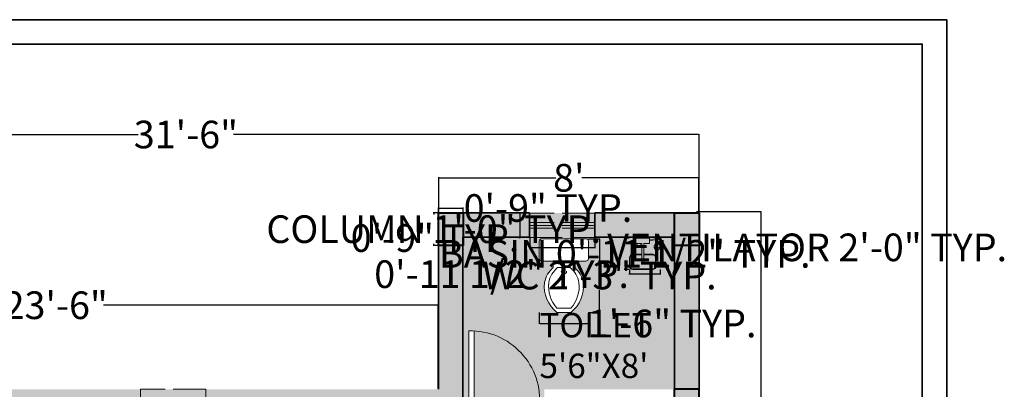
# Model space of a CAD drawing. Units: inches. Extents: x 1077 to 2505, y 1892 to 2728.
# Tile 18 of 26: x 1306 to 1669, y 2586 to 2722. Entities that reach past the tile are written whole.
import ezdxf

# ---------------------------------------------------------------- set-up
doc = ezdxf.new("R2010")
doc.units = ezdxf.units.IN
doc.linetypes.add('ACAD_ISO02W100', pattern=[15, 12, -3])
doc.layers.get('Defpoints').update_dxf_attribs({"color": 220, "linetype": 'ACAD_ISO02W100'})
for name, color, linetype, lineweight in [('A-ANNO-DIMS', 2, 'Continuous', 18), ('A-ANNO-TTLB', 7, 'Continuous', 35), ('A-AREA-IDEN', 7, 'Continuous', 18), ('A-COLS', 7, 'Continuous', 40), ('A-DOOR', 4, 'Continuous', 18), ('A-FLOR-FIXT', 8, 'Continuous', 13), ('A-GLAZ-VENT', 6, 'ACAD_ISO02W100', 13), ('A-WALL-PATT', 7, 'Continuous', 9), ('A_FUR 1', 5, 'Continuous', 5), ('WALL', 7, 'Continuous', 35)]:
    doc.layers.add(name, color=color, linetype=linetype, lineweight=lineweight)
doc.layers.add('A-FLOR-PATT', color=254, linetype='Continuous', lineweight=9, true_color=0xd7ebd2)
doc.styles.get("Standard").update_dxf_attribs({"font": 'arial.ttf'})
doc.dimstyles.get("Standard").update_dxf_attribs({"dimtxt": 10.18, "dimasz": 0.18, "dimexe": 0.18, "dimexo": 0.0625, "dimgap": 0.09, "dimtad": 0, "dimtih": 1, "dimtoh": 1, "dimdec": 0, "dimzin": 0, "dimdsep": 46, "dimlunit": 3, "dimtxsty": 'Standard', "dimcen": 0.09, "dimadec": 0, "dimazin": 0, "dimtfac": 1, "dimtdec": 0, "dimtofl": 0, "dimtmove": 0, "dimatfit": 3, "dimfxl": 1, "dimtolj": 1, "dimtzin": 0, "dimarcsym": 0})

# ---------------------------------------------------------------- blocks, each defined once
blk = doc.blocks.new('*D1')
at = {"layer": 'A-ANNO-DIMS', "color": 0, "lineweight": -2, "transparency": 16777216}
for p, q in [((1460.66, 2651.34), (1460.66, 2664.26)), ((1460.84, 2664.08), (1503.8, 2664.08)), ((1556.32, 2664.08), (1513.36, 2664.08)), ((1556.5, 2651.34), (1556.5, 2664.26))]:
    blk.add_line(p, q, dxfattribs=at)
at = {"layer": 'A-ANNO-DIMS', "color": 0, "transparency": 16777216}
for points in [[(1460.84, 2664.11), (1460.84, 2664.05), (1460.66, 2664.08)], [(1556.32, 2664.11), (1556.32, 2664.05), (1556.5, 2664.08)]]:
    blk.add_solid(points, dxfattribs=at)
at = {"layer": 'Defpoints', "color": 0, "transparency": 16777216}
for p in [(1556.5, 2664.08), (1460.66, 2651.28), (1556.5, 2651.28)]:
    blk.add_point(p, dxfattribs=at)
at = {"layer": 'A-ANNO-DIMS', "color": 0, "transparency": 16777216, "insert": (1508.58, 2664.08), "char_height": 10.18, "attachment_point": 5}
blk.add_mtext("\\A1;8'", dxfattribs=at)
blk = doc.blocks.new('ESTSET')
at = {"layer": 'A_FUR 1'}
for p, q in [((-10.44, 4.1), (-10.44, 32.1)), ((-8.44, 4.1), (-8.44, 32.1)), ((-36.44, 6.1), (-36.44, 3.1)), ((-34.44, 6.1), (-36.44, 6.1)), ((-34.44, 4.1), (-34.44, 6.1)), ((-34.44, 4.1), (-34.44, 6.1)), ((-32.44, 4.1), (-34.44, 4.1)), ((-32.44, 4.1), (-34.44, 4.1)), ((-32.44, 3.1), (-32.44, 4.1)), ((-10.44, 3.1), (-10.44, 4.1)), ((-10.44, 4.1), (-8.44, 4.1)), ((-10.44, 4.1), (-8.44, 4.1)), ((-8.44, 4.1), (-8.44, 6.1)), ((-8.44, 6.1), (-6.44, 6.1)), ((-8.44, 4.1), (-8.44, 6.1)), ((-6.44, 6.1), (-6.44, 3.1)), ((-6.44, 2.1), (-36.44, 2.1)), ((-35.44, 2.1), (-33.44, 2.1)), ((-7.44, 2.1), (-9.44, 2.1))]:
    blk.add_line(p, q, dxfattribs=at)
for points in [[(-21.44, 2.1), (-18.67, 2.1), (-18.67, 5.1), (-20.06, 5.1)], [(-20.06, 5.1), (-20.06, -0.91)], [(-21.44, 2.1), (-21.44, -0.91), (-20.06, -0.91)]]:
    blk.add_lwpolyline(points, dxfattribs=at)
for centre, radius, start, end in [((-8.91, 6.46), 25.64, 88.9606, 185.2816), ((-35.44, 3.1), 1, 180, 270), ((-33.44, 3.1), 1, 270, 0), ((-9.44, 3.1), 1, 180, 270), ((-7.44, 3.1), 1, 270, 0)]:
    blk.add_arc(centre, radius, start, end, dxfattribs=at)
blk = doc.blocks.new('A$C2AC94788')
for p, q in [((0, 0.505), (0, 0.665)), ((0.025, 0.69), (0.435, 0.69)), ((0.46, 0.665), (0.46, 0.505)), ((0.435, 0.48), (0.025, 0.48)), ((0.13, 0.48), (0.13, 0.42)), ((0.33, 0.42), (0.33, 0.48)), ((0.17, 0.42), (0.29, 0.42)), ((0.1641, 0.0392), (0.2959, 0.0392)), ((0.2291, 0.0392), (0.23, 0.0392)), ((0.2309, 0.0392), (0.23, 0.0392)), ((0.165, 0), (0.295, 0))]:
    blk.add_line(p, q)
for centre, radius, start, end in [((0.025, 0.665), 0.025, 90, 180), ((0.435, 0.665), 0.025, 0, 90), ((0.025, 0.505), 0.025, 180, 270), ((0.435, 0.505), 0.025, 270, 0), ((0.2874, 0.2356), 0.2425, 130.48854, 169.44501), ((0.3274, 0.2356), 0.2425, 130.48854, 169.44501), ((0.23, 0.385), 0.025, 180, 0), ((0.1326, 0.2356), 0.2425, 10.55499, 49.51146), ((0.1726, 0.2356), 0.2425, 10.55499, 49.51146), ((0.3601, 0.2448), 0.313, 173.53688, 231.44828), ((0.4001, 0.2448), 0.313, 173.53688, 221.06038), ((0.0999, 0.2448), 0.313, 308.55172, 6.46312), ((0.0599, 0.2448), 0.313, 318.93962, 6.46312)]:
    blk.add_arc(centre, radius, start, end)
blk = doc.blocks.new('A$C7A0926BE')
for p, q in [((-6.55, 0), (-5.57, 0)), ((-6.55, -0.65), (-6.55, 0)), ((-5.57, 0), (-5.57, -0.65)), ((-2.89, 0), (-2.89, -2.29)), ((2.89, 0), (-2.89, 0)), ((2.89, -2.29), (2.89, 0)), ((-7.32, -3.29), (-7.32, -3.94)), ((-5.57, -0.65), (-6.55, -0.65)), ((-6.34, -0.65), (-5.74, -0.65)), ((-6.34, -2.33), (-6.34, -0.65)), ((-5.74, -2.33), (-6.34, -2.33)), ((-5.74, -0.65), (-5.74, -2.33)), ((-5.57, -0.28), (-2.89, -0.56)), ((-5.57, -0.65), (-2.89, -0.94)), ((-4.84, -3.94), (-4.85, -3.29)), ((-2.89, -2.29), (-0.45, -2.29)), ((0.39, -2.29), (2.89, -2.29)), ((1.04, -2.29), (1.04, -3.12)), ((2.37, -2.29), (1.04, -2.29)), ((1.04, -3.12), (2.37, -3.12)), ((1.13, -3.12), (1.13, -3.23)), ((2.3, -3.12), (1.13, -3.12)), ((1.13, -3.23), (2.3, -3.23)), ((2.3, -3.23), (2.3, -3.12)), ((2.37, -3.12), (2.37, -2.29))]:
    blk.add_line(p, q)
at = {"ltscale": 100}
for p, q in [((-0.45, -10.48), (-0.45, -2.29)), ((0.39, -10.48), (0.39, -2.29)), ((0.18, -10.69), (-0.24, -10.69))]:
    blk.add_line(p, q, dxfattribs=at)
for points in [[(-0.45, -6.79), (-4.23, -6.79, 0.414214), (-5.63, -8.19), (-5.63, -11.8, 0.414214), (-4.23, -13.2), (4.17, -13.2, 0.414214), (5.57, -11.8), (5.57, -8.19, 0.414214), (4.17, -6.79), (0.39, -6.79)], [(-0.45, -7), (-4.23, -7, 0.414214), (-5.42, -8.19), (-5.42, -11.8, 0.414214), (-4.23, -12.99), (4.17, -12.99, 0.414214), (5.36, -11.8), (5.36, -8.19, 0.414214), (4.17, -7), (0.39, -7)]]:
    blk.add_lwpolyline(points, format="xyb", dxfattribs=at)
for centre, start, end in [((-0.24, -10.48), 180, 270), ((0.18, -10.48), 270, 0)]:
    blk.add_arc(centre, 0.21, start, end, dxfattribs=at)
at = {"extrusion": (0, 0, -1)}
blk.add_ellipse((-6.08, -3.29), major_axis=(-1.24, 0), ratio=0.790849, dxfattribs=at)
blk.add_ellipse((-6.08, -3.94), major_axis=(-1.24, 0), ratio=0.790849, start_param=3.141593, end_param=6.283185, dxfattribs=at)
blk = doc.blocks.new('C1')
h = blk.add_hatch(color=256)
h.dxf.hatch_style = 1
h.paths.add_polyline_path([(1668.56, 2445.41), (1677.56, 2445.41), (1677.56, 2457.41), (1668.56, 2457.41)])
for p, q in [((1668.56, 2457.41), (1677.56, 2457.41)), ((1668.56, 2445.41), (1668.56, 2457.41)), ((1677.56, 2457.41), (1677.56, 2445.41)), ((1677.56, 2445.41), (1668.56, 2445.41))]:
    blk.add_line(p, q)
blk = doc.blocks.new('*D13')
at = {"layer": 'A-ANNO-DIMS', "color": 0, "lineweight": -2, "transparency": 16777216}
for p, q in [((1178.64, 2586.44), (1178.64, 2617.31)), ((1178.82, 2617.13), (1301.91, 2617.13)), ((1460.32, 2617.13), (1337.23, 2617.13)), ((1460.5, 2586.44), (1460.5, 2617.31))]:
    blk.add_line(p, q, dxfattribs=at)
at = {"layer": 'A-ANNO-DIMS', "color": 0, "transparency": 16777216}
for points in [[(1178.82, 2617.16), (1178.82, 2617.1), (1178.64, 2617.13)], [(1460.32, 2617.16), (1460.32, 2617.1), (1460.5, 2617.13)]]:
    blk.add_solid(points, dxfattribs=at)
at = {"layer": 'Defpoints', "color": 0, "transparency": 16777216}
for p in [(1460.5, 2617.13), (1178.64, 2586.38), (1460.5, 2586.38)]:
    blk.add_point(p, dxfattribs=at)
at = {"layer": 'A-ANNO-DIMS', "color": 0, "transparency": 16777216, "insert": (1319.57, 2617.13), "char_height": 10.18, "attachment_point": 5}
blk.add_mtext('\\A1;23\'-6"', dxfattribs=at)
blk = doc.blocks.new('*D14')
at = {"layer": 'A-ANNO-DIMS', "color": 0, "lineweight": -2, "transparency": 16777216}
for p, q in [((1555.59, 2651.66), (1579.43, 2651.66)), ((1579.25, 2651.48), (1579.25, 2375.3)), ((1579.25, 2088.54), (1579.25, 2364.72)), ((1555.59, 2088.36), (1579.43, 2088.36))]:
    blk.add_line(p, q, dxfattribs=at)
at = {"layer": 'A-ANNO-DIMS', "color": 0, "transparency": 16777216}
for points in [[(1579.22, 2651.48), (1579.28, 2651.48), (1579.25, 2651.66)], [(1579.22, 2088.54), (1579.28, 2088.54), (1579.25, 2088.36)]]:
    blk.add_solid(points, dxfattribs=at)
at = {"layer": 'Defpoints', "color": 0, "transparency": 16777216}
for p in [(1555.53, 2651.66), (1555.53, 2088.36), (1579.25, 2088.36)]:
    blk.add_point(p, dxfattribs=at)
at = {"layer": 'A-ANNO-DIMS', "color": 0, "transparency": 16777216, "insert": (1579.25, 2370.01), "char_height": 10.18, "attachment_point": 5}
blk.add_mtext('\\A1;46\'-11"', dxfattribs=at)
blk = doc.blocks.new('VENT-24')
for p, q in [((3.5, 24), (3.5, 0)), ((4.5, 24), (4.5, 0)), ((5.5, 24), (5.5, 0))]:
    blk.add_line(p, q)
blk.add_lwpolyline([(0, 0), (9, 0), (9, 24), (0, 24)], close=True)
blk = doc.blocks.new('SHEET-FRAME-RESIDENTIAL')
for points in [[(0, 830.04), (543.52, 830.04), (543.52, 0), (0, 0)], [(9, 821.04), (534.52, 821.04), (534.52, 9), (9, 9)]]:
    blk.add_lwpolyline(points, close=True)
blk = doc.blocks.new('*D30')
at = {"layer": 'A-ANNO-DIMS', "color": 0, "lineweight": -2, "transparency": 16777216}
for p, q in [((1460.54, 2651.14), (1458.62, 2651.14)), ((1458.8, 2650.96), (1458.8, 2650.5)), ((1460.54, 2639.14), (1458.62, 2639.14)), ((1458.8, 2639.32), (1458.8, 2639.78))]:
    blk.add_line(p, q, dxfattribs=at)
at = {"layer": 'A-ANNO-DIMS', "color": 0, "transparency": 16777216}
for points in [[(1458.77, 2650.96), (1458.83, 2650.96), (1458.8, 2651.14)], [(1458.77, 2639.32), (1458.83, 2639.32), (1458.8, 2639.14)]]:
    blk.add_solid(points, dxfattribs=at)
at = {"layer": 'Defpoints', "color": 0, "transparency": 16777216}
for p in [(1458.8, 2651.14), (1460.6, 2651.14), (1460.6, 2639.14)]:
    blk.add_point(p, dxfattribs=at)
at = {"layer": 'A-ANNO-DIMS', "color": 0, "transparency": 16777216, "insert": (1458.8, 2645.14), "char_height": 10.18, "attachment_point": 5}
blk.add_mtext('\\A1;COLUMN 1\'-0" TYP.', dxfattribs=at)
blk = doc.blocks.new('*D31')
at = {"layer": 'A-ANNO-DIMS', "color": 0, "lineweight": -2, "transparency": 16777216}
for p, q in [((1460.6, 2651.2), (1460.6, 2653.12)), ((1460.78, 2652.94), (1469.42, 2652.94)), ((1469.6, 2651.2), (1469.6, 2653.12)), ((1469.6, 2652.94), (1469.78, 2652.94))]:
    blk.add_line(p, q, dxfattribs=at)
at = {"layer": 'A-ANNO-DIMS', "color": 0, "transparency": 16777216}
for points in [[(1460.78, 2652.97), (1460.78, 2652.91), (1460.6, 2652.94)], [(1469.42, 2652.97), (1469.42, 2652.91), (1469.6, 2652.94)]]:
    blk.add_solid(points, dxfattribs=at)
at = {"layer": 'Defpoints', "color": 0, "transparency": 16777216}
for p in [(1469.6, 2652.94), (1460.6, 2651.14), (1469.6, 2651.14)]:
    blk.add_point(p, dxfattribs=at)
at = {"layer": 'A-ANNO-DIMS', "color": 0, "transparency": 16777216, "insert": (1500.89, 2652.94), "char_height": 10.18, "attachment_point": 5}
blk.add_mtext('\\A1;0\'-9" TYP.', dxfattribs=at)
blk = doc.blocks.new('*D42')
at = {"layer": 'A-ANNO-DIMS', "color": 0, "lineweight": -2, "transparency": 16777216}
for p, q in [((1515.87, 2641.64), (1520.06, 2641.64)), ((1519.88, 2641.46), (1519.88, 2633.41)), ((1519.88, 2614.65), (1519.88, 2622.7)), ((1515.87, 2614.47), (1520.06, 2614.47))]:
    blk.add_line(p, q, dxfattribs=at)
at = {"layer": 'A-ANNO-DIMS', "color": 0, "transparency": 16777216}
for points in [[(1519.85, 2641.46), (1519.91, 2641.46), (1519.88, 2641.64)], [(1519.85, 2614.65), (1519.91, 2614.65), (1519.88, 2614.47)]]:
    blk.add_solid(points, dxfattribs=at)
at = {"layer": 'Defpoints', "color": 0, "transparency": 16777216}
for p in [(1515.81, 2641.64), (1519.88, 2641.64), (1515.81, 2614.47)]:
    blk.add_point(p, dxfattribs=at)
at = {"layer": 'A-ANNO-DIMS', "color": 0, "transparency": 16777216, "insert": (1519.88, 2628.06), "char_height": 10.18, "attachment_point": 5}
blk.add_mtext('\\A1;WC 2\'-3" TYP.', dxfattribs=at)
blk = doc.blocks.new('*D43')
at = {"layer": 'A-ANNO-DIMS', "color": 0, "lineweight": -2, "transparency": 16777216}
for p, q in [((1497.7, 2614.41), (1497.7, 2610.22)), ((1515.81, 2614.41), (1515.81, 2610.22)), ((1497.88, 2610.4), (1515.63, 2610.4)), ((1515.81, 2610.4), (1515.99, 2610.4))]:
    blk.add_line(p, q, dxfattribs=at)
at = {"layer": 'A-ANNO-DIMS', "color": 0, "transparency": 16777216}
for points in [[(1497.88, 2610.43), (1497.88, 2610.37), (1497.7, 2610.4)], [(1515.63, 2610.43), (1515.63, 2610.37), (1515.81, 2610.4)]]:
    blk.add_solid(points, dxfattribs=at)
at = {"layer": 'Defpoints', "color": 0, "transparency": 16777216}
for p in [(1497.7, 2614.47), (1515.81, 2614.47), (1515.81, 2610.4)]:
    blk.add_point(p, dxfattribs=at)
at = {"layer": 'A-ANNO-DIMS', "color": 0, "transparency": 16777216, "insert": (1546.63, 2610.4), "char_height": 10.18, "attachment_point": 5}
blk.add_mtext('\\A1;1\'-6" TYP.', dxfattribs=at)
blk = doc.blocks.new('*D52')
at = {"layer": 'A-ANNO-DIMS', "color": 0, "lineweight": -2, "transparency": 16777216}
for p, q in [((1530.85, 2641.82), (1529, 2641.82)), ((1529.18, 2641.64), (1529.18, 2641.42)), ((1530.85, 2630.3), (1529, 2630.3)), ((1529.18, 2630.48), (1529.18, 2630.71))]:
    blk.add_line(p, q, dxfattribs=at)
at = {"layer": 'A-ANNO-DIMS', "color": 0, "transparency": 16777216}
for points in [[(1529.15, 2641.64), (1529.21, 2641.64), (1529.18, 2641.82)], [(1529.15, 2630.48), (1529.21, 2630.48), (1529.18, 2630.3)]]:
    blk.add_solid(points, dxfattribs=at)
at = {"layer": 'Defpoints', "color": 0, "transparency": 16777216}
for p in [(1529.18, 2641.82), (1530.91, 2641.82), (1530.91, 2630.3)]:
    blk.add_point(p, dxfattribs=at)
at = {"layer": 'A-ANNO-DIMS', "color": 0, "transparency": 16777216, "insert": (1529.18, 2636.06), "char_height": 10.18, "attachment_point": 5}
blk.add_mtext('\\A1;BASIN 0\'-11 1/2" TYP.', dxfattribs=at)
blk = doc.blocks.new('*D53')
at = {"layer": 'A-ANNO-DIMS', "color": 0, "lineweight": -2, "transparency": 16777216}
for p, q in [((1530.91, 2630.24), (1530.91, 2628.39)), ((1542.17, 2630.24), (1542.17, 2628.39)), ((1530.91, 2628.57), (1530.73, 2628.57)), ((1541.99, 2628.57), (1531.09, 2628.57))]:
    blk.add_line(p, q, dxfattribs=at)
at = {"layer": 'A-ANNO-DIMS', "color": 0, "transparency": 16777216}
for points in [[(1531.09, 2628.6), (1531.09, 2628.54), (1530.91, 2628.57)], [(1541.99, 2628.6), (1541.99, 2628.54), (1542.17, 2628.57)]]:
    blk.add_solid(points, dxfattribs=at)
at = {"layer": 'Defpoints', "color": 0, "transparency": 16777216}
for p in [(1530.91, 2630.3), (1542.17, 2630.3), (1530.91, 2628.57)]:
    blk.add_point(p, dxfattribs=at)
at = {"layer": 'A-ANNO-DIMS', "color": 0, "transparency": 16777216, "insert": (1483.8, 2628.57), "char_height": 10.18, "attachment_point": 5}
blk.add_mtext('\\A1;0\'-11 1/2" TYP.', dxfattribs=at)
blk = doc.blocks.new('*D60')
at = {"layer": 'A-ANNO-DIMS', "color": 0, "lineweight": -2, "transparency": 16777216}
for p, q in [((1494.18, 2641.99), (1494.18, 2638.27)), ((1518.18, 2641.99), (1518.18, 2638.27)), ((1494.36, 2638.45), (1518, 2638.45)), ((1518.18, 2638.45), (1518.36, 2638.45))]:
    blk.add_line(p, q, dxfattribs=at)
at = {"layer": 'A-ANNO-DIMS', "color": 0, "transparency": 16777216}
for points in [[(1494.36, 2638.48), (1494.36, 2638.42), (1494.18, 2638.45)], [(1518, 2638.48), (1518, 2638.42), (1518.18, 2638.45)]]:
    blk.add_solid(points, dxfattribs=at)
at = {"layer": 'Defpoints', "color": 0, "transparency": 16777216}
for p in [(1494.18, 2642.05), (1518.18, 2642.05), (1518.18, 2638.45)]:
    blk.add_point(p, dxfattribs=at)
at = {"layer": 'A-ANNO-DIMS', "color": 0, "transparency": 16777216, "insert": (1596.37, 2638.45), "char_height": 10.18, "attachment_point": 5}
blk.add_mtext('\\A1;VENTILATOR 2\'-0" TYP.', dxfattribs=at)
blk = doc.blocks.new('*D61')
at = {"layer": 'A-ANNO-DIMS', "color": 0, "lineweight": -2, "transparency": 16777216}
for p, q in [((1494.12, 2651.05), (1490.4, 2651.05)), ((1490.58, 2650.87), (1490.58, 2642.23)), ((1494.12, 2642.05), (1490.4, 2642.05)), ((1490.58, 2641.87), (1490.4, 2641.87)), ((1490.58, 2642.05), (1490.58, 2641.87))]:
    blk.add_line(p, q, dxfattribs=at)
at = {"layer": 'A-ANNO-DIMS', "color": 0, "transparency": 16777216}
for points in [[(1490.55, 2650.87), (1490.61, 2650.87), (1490.58, 2651.05)], [(1490.55, 2642.23), (1490.61, 2642.23), (1490.58, 2642.05)]]:
    blk.add_solid(points, dxfattribs=at)
at = {"layer": 'Defpoints', "color": 0, "transparency": 16777216}
for p in [(1494.18, 2651.05), (1490.58, 2642.05), (1494.18, 2642.05)]:
    blk.add_point(p, dxfattribs=at)
at = {"layer": 'A-ANNO-DIMS', "color": 0, "transparency": 16777216, "insert": (1459.29, 2641.87), "char_height": 10.18, "attachment_point": 5}
blk.add_mtext('\\A1;0\'-9" TYP.', dxfattribs=at)
blk = doc.blocks.new('*D62')
at = {"layer": 'A-ANNO-DIMS', "color": 0, "lineweight": -2, "transparency": 16777216}
for p, q in [((1178.53, 2586.22), (1178.53, 2680.19)), ((1178.71, 2680.01), (1349.96, 2680.01)), ((1556.35, 2680.01), (1385.1, 2680.01)), ((1556.53, 2651.22), (1556.53, 2680.19))]:
    blk.add_line(p, q, dxfattribs=at)
at = {"layer": 'A-ANNO-DIMS', "color": 0, "transparency": 16777216}
for points in [[(1178.71, 2680.04), (1178.71, 2679.98), (1178.53, 2680.01)], [(1556.35, 2680.04), (1556.35, 2679.98), (1556.53, 2680.01)]]:
    blk.add_solid(points, dxfattribs=at)
at = {"layer": 'Defpoints', "color": 0, "transparency": 16777216}
for p in [(1556.53, 2680.01), (1556.53, 2651.16), (1178.53, 2586.16)]:
    blk.add_point(p, dxfattribs=at)
at = {"layer": 'A-ANNO-DIMS', "color": 0, "transparency": 16777216, "insert": (1367.53, 2680.01), "char_height": 10.18, "attachment_point": 5}
blk.add_mtext('\\A1;31\'-6"', dxfattribs=at)

msp = doc.modelspace()

# ---------------------------------------------------------------- hatches: boundary and pattern name
at = {"layer": 'A-FLOR-PATT', "transparency": 33554559}
h = msp.add_hatch(color=256, dxfattribs=at)
h.dxf.hatch_style = 1
h.paths.add_polyline_path([(1395.53, 2577.16), (1374.83, 2577.16), (1350.83, 2577.19), (1350.83, 2577.16), (1329.53, 2577.16), (1329.53, 2480.16), (1329.53, 2469.16), (1325.53, 2469.16), (1325.53, 2515.13), (1307.53, 2515.13), (1307.53, 2577.16), (1269.31, 2577.16), (1221.31, 2577.15), (1221.31, 2577.16), (1187.53, 2577.16), (1187.53, 2433.16), (1289.53, 2433.16), (1289.53, 2429.16), (1263.53, 2429.16), (1187.53, 2429.16), (1187.53, 2395.02), (1187.53, 2395.02), (1187.53, 2371.02), (1187.53, 2371.02), (1187.53, 2307.16), (1259.53, 2307.16), (1259.53, 2399.16), (1263.53, 2399.16), (1263.53, 2307.16), (1289.53, 2307.16), (1289.53, 2306.23), (1325.53, 2306.23), (1325.53, 2307.16), (1329.53, 2307.16), (1329.53, 2306.23), (1365.53, 2306.23), (1365.53, 2307.16), (1432.53, 2307.16), (1432.53, 2088.16), (1547.53, 2088.16), (1547.53, 2140.08), (1511.53, 2140.08), (1511.53, 2267.16), (1475.53, 2267.16), (1475.53, 2303.16), (1468.53, 2303.16), (1468.53, 2307.16), (1547.53, 2307.16), (1547.53, 2348.22), (1547.53, 2396.22), (1547.53, 2429.16), (1435.53, 2429.16), (1435.53, 2433.16), (1476.35, 2433.16), (1476.35, 2451.18), (1547.53, 2451.18), (1547.53, 2577.16), (1499.53, 2577.16), (1499.53, 2586.16), (1547.53, 2586.16), (1547.53, 2642.16), (1518.18, 2642.16), (1518.18, 2642.05), (1494.15, 2642.05), (1494.15, 2642.16), (1469.53, 2642.16), (1469.53, 2577.16), (1399.53, 2577.16), (1399.53, 2429.16), (1325.53, 2429.16), (1325.53, 2433.16), (1329.53, 2433.16), (1395.53, 2433.16), (1395.53, 2480.16), (1359.53, 2480.16), (1359.53, 2484.16), (1395.53, 2484.16)])
h.paths.add_polyline_path([(1357.65, 2482.07), (1355.65, 2482.07), (1355.65, 2481.07, 0.414214), (1356.65, 2480.07), (1344.65, 2480.07), (1344.65, 2477.06), (1343.27, 2477.06), (1343.27, 2480.07), (1330.65, 2480.07, -0.414214), (1329.65, 2481.07), (1329.65, 2484.07), (1331.65, 2484.07), (1331.65, 2510.07, -0.446908)], flags=16)
h.paths.add_polyline_path([(1305.09, 2559.18), (1288.89, 2559.18), (1288.89, 2575.38), (1305.09, 2575.38)], flags=16)
h.paths.add_polyline_path([(1304.19, 2560.08), (1289.79, 2560.08), (1289.79, 2574.48), (1304.19, 2574.48)], flags=0)
h.paths.add_polyline_path([(1287.99, 2500.68, -0.414214), (1287.09, 2499.78), (1265.14, 2499.78), (1224.09, 2499.78, -0.414214), (1223.19, 2500.68), (1223.19, 2557.16), (1223.19, 2571.74), (1223.19, 2575.38), (1287.99, 2575.38), (1287.99, 2571.74), (1287.09, 2571.74, -0.414214), (1287.99, 2570.84)], flags=16)
h.paths.add_polyline_path([(1292.98, 2569.05, -1), (1300.92, 2569.05, -1)], flags=0)
h.paths.add_polyline_path([(1293.32, 2569.05, -1), (1300.58, 2569.05, -1)], flags=0)
h.paths.add_polyline_path([(1322.8, 2462.21), (1322.8, 2431.71), (1323.05, 2430.71), (1323.05, 2431.71), (1321.8, 2431.71), (1321.8, 2462.19, 0.404641), (1292.3, 2431.71), (1292.05, 2430.71, -0.414214), (1291.55, 2430.21), (1291.05, 2430.21), (1291.05, 2429.71, -0.414214), (1290.55, 2429.21), (1289.55, 2429.21), (1289.55, 2434.21), (1290.55, 2434.21, -0.414214), (1291.05, 2433.71), (1291.05, 2433.21), (1291.55, 2433.21, -0.414214), (1292.05, 2432.71), (1292.3, 2431.71, -0.414214)], flags=16)
h.paths.add_polyline_path([(1287.82, 2548.28, 0.292232), (1279.17, 2536.8, 0.052719), (1223.93, 2548.28), (1223.28, 2548.28), (1223.28, 2557.16), (1223.93, 2557.16), (1245.42, 2557.16, -0.117785), (1245.77, 2557.93, -0.059418), (1254.87, 2567.02, -0.379859), (1257.28, 2566.88, -0.02509), (1261.41, 2563.32, -0.025935), (1265.65, 2567.02, -0.379859), (1268.06, 2566.88, -0.061767), (1277.52, 2557.43, -0.069393), (1277.82, 2557.16), (1287.82, 2557.16)], flags=0)
h.paths.add_polyline_path([(1263.47, 2548.28), (1260.56, 2548.28, -0.015371), (1258.01, 2546.13, -0.429576), (1255.37, 2546.06, -0.016036), (1252.69, 2548.28), (1223.28, 2548.28), (1223.28, 2554.42), (1246.78, 2554.42, 0.055344), (1255.37, 2546.06, 0.331768), (1257.52, 2545.74, 0.027343), (1262, 2549.64, 0.00919)], flags=0)
h.paths.add_polyline_path([(1295.56, 2568.34), (1296.87, 2569.09), (1296.87, 2570.6, 0.399698), (1295.39, 2569.05, 0.119004)], flags=0)
h.paths.add_polyline_path([(1295.21, 2569.05, -1), (1298.68, 2569.05, -1)], flags=0)
h.paths.add_polyline_path([(1296.95, 2568.96), (1297.03, 2569), (1297.03, 2569.09), (1296.99, 2569.11), (1296.91, 2568.98)], flags=0)
h.paths.add_polyline_path([(1402.28, 2462.19, -0.414214), (1432.78, 2431.69), (1433.03, 2432.69), (1432.78, 2431.69, 0.404641), (1403.28, 2462.17), (1403.28, 2431.69), (1402.03, 2431.69), (1402.03, 2430.69, -0.414214), (1401.53, 2430.19), (1401.03, 2430.19), (1401.03, 2429.69, -0.414214), (1400.53, 2429.19), (1399.53, 2429.19), (1399.53, 2434.19), (1400.53, 2434.19, -0.414214), (1401.03, 2433.69), (1401.03, 2433.19), (1401.53, 2433.19, -0.414214), (1402.03, 2432.69)], flags=16)
h.paths.add_polyline_path([(1470.16, 2535.21, -0.414214), (1471.06, 2536.11), (1527.54, 2536.11), (1542.12, 2536.11), (1545.76, 2536.11), (1545.76, 2471.31), (1542.12, 2471.31), (1542.12, 2472.21, -0.414214), (1541.22, 2471.31), (1471.06, 2471.31, -0.414214), (1470.16, 2472.21), (1470.16, 2494.16)], flags=16)
h.paths.add_polyline_path([(1483.07, 2536.11, 0.253465), (1480.11, 2526.15, 0.2538), (1470.15, 2523.19)], flags=16)
h.paths.add_polyline_path([(1223.19, 2512.69, 0.253465), (1233.14, 2509.74, 0.2538), (1236.1, 2499.77)], flags=16)
h.paths.add_polyline_path([(1469.77, 2578.72), (1469.77, 2581.72), (1471.77, 2581.72), (1471.77, 2607.72, -0.01951), (1473.77, 2607.68), (1473.77, 2579.72), (1473.77, 2578.72, -0.414214), (1472.77, 2577.72), (1470.77, 2577.72, -0.414214)], flags=16)
h.paths.add_polyline_path([(1382.46, 2398.13), (1395.04, 2398.13), (1395.04, 2399.74), (1382.46, 2399.74)], flags=16)
h.paths.add_polyline_path([(1379.94, 2397.18), (1379.94, 2389.82), (1380.5, 2389.82), (1380.5, 2396.05, -0.41429), (1381.06, 2396.61), (1396.47, 2396.61, -0.414213), (1397.03, 2396.05), (1397.03, 2389.82), (1397.59, 2389.82), (1397.59, 2397.18)], flags=16)
h.paths.add_polyline_path([(1263.37, 2428.14), (1263.37, 2426.14, -0.414214), (1262.37, 2425.14), (1261.37, 2425.14), (1233.41, 2425.14, 0.400854), (1259.37, 2401.04), (1259.37, 2401.14), (1261.37, 2401.14, -0.446908), (1233.37, 2427.14), (1259.37, 2427.14), (1259.37, 2429.14), (1262.37, 2429.14, -0.414214)], flags=16)
h.paths.add_polyline_path([(1404.79, 2398.13), (1417.37, 2398.13), (1417.37, 2399.74), (1404.79, 2399.74)], flags=16)
h.paths.add_polyline_path([(1402.27, 2397.18), (1404.79, 2398.13), (1417.37, 2398.13), (1419.92, 2397.18)], flags=16)
h.paths.add_polyline_path([(1432.26, 2383.16), (1432.26, 2370.59), (1433.87, 2370.59), (1433.87, 2383.16)], flags=16)
h.paths.add_polyline_path([(1431.3, 2385.69), (1423.84, 2385.69), (1423.84, 2385.13), (1430.18, 2385.13, -0.41429), (1430.74, 2384.57), (1430.74, 2369.16, -0.414237), (1430.18, 2368.6), (1423.84, 2368.6), (1423.84, 2368.03), (1431.3, 2368.03)], flags=16)
h.paths.add_polyline_path([(1417.37, 2351.16), (1417.37, 2349.54), (1418.9, 2349.54, 0.414236), (1419.92, 2350.56), (1419.92, 2352.11)], flags=16)
h.paths.add_polyline_path([(1395.04, 2351.16), (1395.04, 2349.54), (1396.58, 2349.54, 0.414235), (1397.59, 2350.56), (1397.59, 2352.11)], flags=16)
h.paths.add_polyline_path([(1366.7, 2370.05), (1365.09, 2370.05), (1365.09, 2368.52, 0.414235), (1366.11, 2367.5), (1367.66, 2367.5)], flags=16)
h.paths.add_polyline_path([(1419.36, 2359.47), (1419.36, 2353.24, -0.41419), (1418.8, 2352.68), (1403.39, 2352.68, -0.414137), (1402.83, 2353.24), (1402.83, 2359.47), (1397.03, 2359.47), (1397.03, 2353.24, -0.414189), (1396.47, 2352.68), (1381.06, 2352.68, -0.414137), (1380.5, 2353.24), (1380.5, 2359.47)], flags=16)
h.paths.add_polyline_path([(1222.29, 2559.18), (1206.09, 2559.18), (1206.09, 2575.38), (1222.29, 2575.38)], flags=16)
h.paths.add_polyline_path([(1221.39, 2560.08), (1206.99, 2560.08), (1206.99, 2574.48), (1221.39, 2574.48)], flags=0)
h.paths.add_polyline_path([(1482, 2577.72), (1482, 2580.73), (1483.38, 2580.73), (1483.38, 2577.72), (1484.77, 2577.72), (1484.77, 2574.72), (1483.38, 2574.72), (1483.38, 2577.72)], flags=16)
h.paths.add_polyline_path([(1266.37, 2415.53), (1266.37, 2414.14), (1263.37, 2414.14), (1263.37, 2415.53), (1260.36, 2415.53), (1260.36, 2416.91), (1263.37, 2416.91), (1263.37, 2415.53)], flags=16)
h.paths.add_polyline_path([(1210.26, 2569.05, -1), (1218.19, 2569.05, -1)], flags=0)
h.paths.add_polyline_path([(1210.6, 2569.05, -1), (1217.85, 2569.05, -1)], flags=0)
h.paths.add_polyline_path([(1212.84, 2568.34), (1214.15, 2569.09), (1214.15, 2570.6, 0.399698), (1212.67, 2569.05, 0.119004)], flags=0)
h.paths.add_polyline_path([(1212.49, 2569.05, -1), (1215.96, 2569.05, -1)], flags=0)
h.paths.add_polyline_path([(1214.23, 2568.96), (1214.3, 2568.91), (1214.3, 2569)], flags=0)
h.paths.add_polyline_path([(1507.18, 2480.12, 0.052719), (1518.66, 2535.36), (1518.66, 2536.01), (1527.54, 2536.01), (1527.54, 2535.36), (1527.54, 2513.88, -0.117785), (1528.31, 2513.53, -0.059418), (1537.4, 2504.43, -0.379859), (1537.26, 2502.01, -0.02509), (1533.7, 2497.89, -0.025935), (1537.4, 2493.64, -0.379859), (1537.26, 2491.23, -0.061767), (1527.8, 2481.77, -0.069393), (1527.54, 2481.47), (1527.54, 2471.47), (1518.66, 2471.47, 0.292232)], flags=0)
h.paths.add_polyline_path([(1516.43, 2503.92, -0.016036), (1518.66, 2506.6), (1518.66, 2536.01), (1524.8, 2536.01), (1524.8, 2512.51, 0.055344), (1516.43, 2503.92, 0.331768), (1516.12, 2501.77, 0.027343), (1520.01, 2497.29, 0.00919), (1518.66, 2495.82), (1518.66, 2498.73, -0.015371), (1516.5, 2501.28, -0.429576)], flags=0)
h.paths.add_polyline_path([(1499.63, 2625.5, -0.171636), (1502.82, 2631.01), (1502.82, 2633.37), (1498.68, 2633.37, -0.414214), (1497.7, 2634.36), (1497.7, 2640.66, -0.414214), (1498.68, 2641.64), (1514.82, 2641.64, -0.414214), (1515.81, 2640.66), (1515.81, 2634.36, -0.414214), (1514.82, 2633.37), (1510.69, 2633.37), (1510.69, 2631.01, -0.171636), (1513.88, 2625.5, -0.258205), (1509.31, 2614.47), (1504.19, 2614.47, -0.258205)], flags=16)
h.paths.add_polyline_path([(1501.2, 2625.5, -0.171636), (1504.39, 2631.01), (1509.12, 2631.01, -0.171636), (1512.3, 2625.5, -0.210384), (1509.35, 2616.02), (1504.16, 2616.02, -0.210384)], flags=0)
h.paths.add_polyline_path([(1529.56, 2537.01), (1529.56, 2553.21), (1545.76, 2553.21), (1545.76, 2537.01)], flags=16)
h.paths.add_polyline_path([(1530.46, 2537.91), (1530.46, 2552.31), (1544.86, 2552.31), (1544.86, 2537.91)], flags=0)
h.paths.add_polyline_path([(1535.45, 2545.07, -1), (1543.39, 2545.07, -1)], flags=0)
h.paths.add_polyline_path([(1535.8, 2545.07, -1), (1543.05, 2545.07, -1)], flags=0)
h.paths.add_polyline_path([(1529.56, 2470.41), (1545.76, 2470.41), (1545.76, 2454.21), (1529.56, 2454.21)], flags=16)
h.paths.add_polyline_path([(1541.16, 2544.99), (1540.98, 2544.99, -0.544606), (1538.71, 2543.68), (1538.62, 2543.53, 0.547962)], flags=0)
h.paths.add_polyline_path([(1530.46, 2469.51), (1544.86, 2469.51), (1544.86, 2455.11), (1530.46, 2455.11)], flags=0)
h.paths.add_polyline_path([(1539.47, 2545.14), (1539.42, 2545.22), (1539.38, 2545.14)], flags=0)
h.paths.add_polyline_path([(1543.39, 2462.34, -1), (1535.45, 2462.34, -1)], flags=0)
h.paths.add_polyline_path([(1543.05, 2462.34, -1), (1535.8, 2462.34, -1)], flags=0)
h.paths.add_polyline_path([(1541.16, 2462.27), (1540.98, 2462.27, -0.544606), (1538.71, 2460.96), (1538.62, 2460.8, 0.547962)], flags=0)
h.paths.add_polyline_path([(1539.47, 2462.42), (1539.42, 2462.5), (1539.38, 2462.42)], flags=0)
h.paths.add_polyline_path([(1435.32, 2335.25, -0.414214), (1465.82, 2304.75), (1466.07, 2305.75), (1465.82, 2304.75, 0.404641), (1436.32, 2335.23), (1436.32, 2304.75), (1435.07, 2304.75), (1435.07, 2303.75, -0.414214), (1434.57, 2303.25), (1434.07, 2303.25), (1434.07, 2302.75, -0.414214), (1433.57, 2302.25), (1432.57, 2302.25), (1432.57, 2307.25), (1433.57, 2307.25, -0.414214), (1434.07, 2306.75), (1434.07, 2306.25), (1434.57, 2306.25, -0.414214), (1435.07, 2305.75)], flags=16)
h.paths.add_polyline_path([(1532.13, 2635.71), (1535.43, 2635.71), (1535.43, 2635.89), (1532.13, 2635.89)], flags=16)
edge = h.paths.add_edge_path(flags=16)
edge.add_arc((1535.98, 2632.67), 0.183, 270, 360)
edge.add_line((1536.17, 2632.67), (1536.17, 2639.82))
edge.add_line((1536.17, 2639.82), (1538.29, 2639.82))
edge.add_line((1538.29, 2639.82), (1538.29, 2641.82))
edge.add_line((1538.29, 2641.82), (1533.25, 2641.82))
edge.add_line((1533.25, 2641.82), (1533.25, 2639.82))
edge.add_line((1533.25, 2639.82), (1534.87, 2639.82))
edge.add_line((1534.87, 2639.82), (1534.87, 2639))
edge.add_line((1534.87, 2639), (1533.7, 2639))
edge.add_line((1533.7, 2639), (1533.7, 2639.82))
edge.add_line((1533.7, 2639.82), (1533.25, 2639.82))
edge.add_line((1533.25, 2639.82), (1533.25, 2641.82))
edge.add_line((1533.25, 2641.82), (1538.29, 2641.82))
edge.add_line((1538.29, 2641.82), (1538.29, 2641.34))
edge.add_line((1538.29, 2641.34), (1540.64, 2641.58))
edge.add_line((1540.64, 2641.58), (1540.64, 2641.82))
edge.add_line((1540.64, 2641.82), (1541.5, 2641.82))
edge.add_line((1541.5, 2641.82), (1541.5, 2641.25))
edge.add_line((1541.5, 2641.25), (1541.31, 2639.79))
edge.add_ellipse((1541.09, 2638.95), major_axis=(-1.08, 0), ratio=0.790849, start_angle=180, end_angle=255.2976, ccw=False)
edge.add_line((1542.17, 2638.95), (1542.17, 2638.38))
edge.add_ellipse((1541.09, 2638.38), major_axis=(-1.08, 0), ratio=0.790849, start_angle=0, end_angle=180, ccw=False)
edge.add_line((1540, 2638.38), (1540.01, 2638.87))
edge.add_ellipse((1541.09, 2638.95), major_axis=(-1.08, 0), ratio=0.790849, start_angle=284.7024, end_angle=364.0401, ccw=False)
edge.add_line((1540.78, 2639.75), (1540.78, 2641.25))
edge.add_line((1540.78, 2641.25), (1540.64, 2641.25))
edge.add_line((1540.64, 2641.25), (1538.29, 2641.01))
edge.add_line((1538.29, 2641.01), (1538.29, 2639.82))
edge.add_line((1538.29, 2639.82), (1536.17, 2639.82))
edge.add_line((1536.17, 2639.82), (1536.17, 2632.48))
edge.add_line((1536.17, 2632.48), (1535.98, 2632.48))
h.paths.add_polyline_path([(1496.32, 2250.34, -0.292371), (1498.9, 2247.83, -0.085148), (1501.21, 2208.85, -0.01331), (1500.27, 2098.5, -0.379287), (1497.22, 2095.28, -0.0502), (1441.54, 2095.28, -0.379287), (1438.5, 2098.5, -0.01331), (1437.56, 2208.85, -0.086132), (1439.96, 2248.26, -0.295116), (1442.59, 2250.78, -0.114238)], flags=16)
h.paths.add_polyline_path([(1495.16, 2205.84, -0.355389), (1496.7, 2202.1), (1492.94, 2189.65, -0.398275), (1489.12, 2187.47, 0.113332), (1449.64, 2187.47, -0.398275), (1445.82, 2189.65), (1442.06, 2202.1, -0.355394), (1443.6, 2205.84, -0.265725)], flags=0)
h.paths.add_polyline_path([(1440.37, 2195.72), (1445.94, 2181.67), (1445.94, 2160.63), (1440.84, 2157.26)], flags=0)
h.paths.add_polyline_path([(1498.46, 2195.72), (1497.99, 2157.26), (1492.88, 2160.63), (1492.88, 2181.67)], flags=0)
h.paths.add_polyline_path([(1445.94, 2158.37), (1445.94, 2137.12), (1441.12, 2122.56), (1440.87, 2155.03)], flags=0)
h.paths.add_polyline_path([(1492.88, 2158.37), (1497.96, 2155.03), (1497.71, 2122.56), (1492.88, 2137.12)], flags=0)
h.paths.add_polyline_path([(1489.88, 2130.4), (1494.39, 2107.67, -0.090102), (1444.44, 2107.65), (1448.95, 2130.39, 0.036636)], flags=0)
h.paths.add_polyline_path([(1447.54, 2159.34), (1497.44, 2159.34), (1497.44, 2177.89), (1447.54, 2177.89)], flags=8)
h.paths.add_polyline_path([(1196.44, 2354.84), (1246.65, 2354.84), (1246.65, 2388.43), (1196.44, 2388.43)], flags=24)
h.paths.add_polyline_path([(1296.09, 2360.25), (1353.81, 2360.25), (1353.81, 2393.84), (1296.09, 2393.84)], flags=24)
h.paths.add_polyline_path([(1400.72, 2471.85), (1470.63, 2471.85), (1470.63, 2505.44), (1400.72, 2505.44)], flags=24)
h.paths.add_polyline_path([(1324.78, 2448.48), (1394.95, 2448.48), (1394.95, 2467.02), (1324.78, 2467.02)], flags=24)
h.paths.add_polyline_path([(1335.08, 2531.43), (1389.67, 2531.43), (1389.67, 2565.02), (1335.08, 2565.02)], flags=24)
h.paths.add_polyline_path([(1225.76, 2460), (1295.67, 2460), (1295.67, 2493.58), (1225.76, 2493.58)], flags=24)
at = {"layer": 'A-WALL-PATT', "transparency": 33554585}
h = msp.add_hatch(color=256, dxfattribs=at)
h.dxf.hatch_style = 1
h.paths.add_polyline_path([(1187.53, 2424), (1178.53, 2424), (1178.53, 2395.02), (1187.53, 2395.02)])
h.paths.add_polyline_path([(1187.53, 2371.02), (1178.53, 2371.02), (1178.53, 2311.49), (1187.53, 2311.49)])
h.paths.add_polyline_path([(1228.13, 2153.16), (1187.53, 2153.16), (1187.53, 2219.66), (1178.53, 2219.66), (1178.53, 2100.18), (1187.53, 2100.18), (1187.53, 2144.16), (1228.13, 2144.16)])
h.paths.add_polyline_path([(1432.53, 2097.16), (1187.53, 2097.16), (1187.53, 2100.18), (1178.53, 2100.18), (1178.53, 2088.16), (1432.53, 2088.16)])
h.paths.add_polyline_path([(1556.53, 2348.22), (1547.53, 2348.22), (1547.53, 2348.22), (1547.53, 2307.16), (1468.53, 2307.16), (1468.53, 2303.16), (1547.53, 2303.16), (1547.53, 2088.16), (1556.53, 2088.16)])
h.paths.add_polyline_path([(1556.53, 2425.11), (1547.53, 2425.11), (1547.53, 2396.22), (1556.53, 2396.22)])
h.paths.add_polyline_path([(1547.53, 2433.16), (1435.53, 2433.16), (1435.53, 2429.16), (1547.53, 2429.16)])
h.paths.add_polyline_path([(1556.53, 2574.38), (1547.53, 2574.38), (1547.53, 2451.18), (1547.55, 2451.18), (1547.55, 2437.11), (1556.53, 2437.11)])
h.paths.add_polyline_path([(1556.53, 2639.11), (1547.53, 2639.11), (1547.53, 2586.38), (1556.53, 2586.38)])
h.paths.add_polyline_path([(1556.53, 2639.11), (1547.53, 2639.11), (1547.53, 2642.16), (1518.18, 2642.16), (1518.18, 2642.05), (1494.18, 2642.05), (1494.18, 2651.05), (1518.15, 2651.05), (1518.15, 2651.16), (1556.53, 2651.16)])
h.paths.add_polyline_path([(1494.15, 2651.16), (1469.6, 2651.16), (1469.6, 2642.16), (1494.15, 2642.16)])
h.paths.add_polyline_path([(1221.31, 2577.16), (1187.61, 2577.16), (1187.61, 2574.03), (1178.61, 2574.03), (1178.61, 2586.16), (1221.31, 2586.16)])
h.paths.add_polyline_path([(1323.07, 2586.16), (1269.31, 2586.16), (1269.31, 2577.16), (1323.07, 2577.16)])
h.paths.add_polyline_path([(1374.84, 2586.19), (1374.84, 2577.19), (1350.84, 2577.19), (1350.83, 2577.19), (1350.83, 2577.16), (1332.07, 2577.16), (1332.07, 2574), (1323.07, 2574), (1323.07, 2586.16), (1350.83, 2586.16), (1350.84, 2586.16), (1350.84, 2586.19)])
h.paths.add_polyline_path([(1392.95, 2586.16), (1374.84, 2586.16), (1374.84, 2577.16), (1392.95, 2577.16)], flags=17)
h.paths.add_polyline_path([(1469.53, 2642.16), (1469.6, 2651.16), (1460.53, 2651.16), (1460.53, 2586.16), (1392.95, 2586.16), (1392.95, 2577.16), (1395.53, 2577.16), (1395.53, 2484.16), (1359.53, 2484.16), (1359.53, 2480.16), (1395.53, 2480.16), (1395.53, 2433.16), (1329.53, 2433.16), (1325.53, 2433.16), (1325.53, 2429.16), (1399.53, 2429.16), (1399.53, 2577.16), (1469.53, 2577.16)])
h.paths.add_polyline_path([(1187.53, 2574.03), (1178.53, 2574.03), (1178.53, 2436), (1187.53, 2436)])

# ---------------------------------------------------------------- linework, layer by layer
at = {"layer": 'WALL'}
for p, q in [((1460.53, 2651.16), (1494.15, 2651.16)), ((1460.53, 2651.16), (1460.53, 2586.16)), ((1494.15, 2642.16), (1494.15, 2651.16)), ((1518.15, 2642.16), (1518.15, 2651.16)), ((1518.15, 2651.16), (1556.53, 2651.16)), ((1556.53, 2651.16), (1556.53, 2396.22)), ((1469.53, 2642.16), (1494.15, 2642.16)), ((1469.53, 2642.16), (1469.53, 2577.16)), ((1518.15, 2642.16), (1547.53, 2642.16)), ((1547.53, 2642.16), (1547.53, 2586.16))]:
    msp.add_line(p, q, dxfattribs=at)

# ---------------------------------------------------------------- block references
at = {"layer": 'A-ANNO-TTLB'}
msp.add_blockref('SHEET-FRAME-RESIDENTIAL', (1104.25, 1892.27), dxfattribs=at)
at = {"layer": 'A-COLS'}
for p in [(-207.96, 193.73), (-121.03, 193.7), (-121.05, 128.98)]:
    msp.add_blockref('C1', p, dxfattribs=at)
at = {"layer": 'A-DOOR', "xscale": -1}
msp.add_blockref('ESTSET', (1463.32, 2575.63), dxfattribs=at)
at = {"layer": 'A-FLOR-FIXT', "xscale": 39.375, "yscale": 39.375, "zscale": 39.375}
msp.add_blockref('A$C2AC94788', (1497.7, 2614.47), dxfattribs=at)
at = {"layer": 'A-FLOR-FIXT', "extrusion": (0, 0, -1), "xscale": 0.8732967133751344, "yscale": 0.8732967133751344, "zscale": -0.8732967133751344}
msp.add_blockref('A$C7A0926BE', (-1535.77, 2641.82), dxfattribs=at)
at = {"layer": 'A-GLAZ-VENT'}
for p, rotation in [((1494.18, 2651.05), 269.9999999999988), ((1350.84, 2586.19), 269.9999999999953)]:
    msp.add_blockref('VENT-24', p, dxfattribs=dict(at, rotation=rotation))

# ---------------------------------------------------------------- texts
at = {"layer": 'A-AREA-IDEN', "insert": (1497.77, 2614.3), "char_height": 9, "attachment_point": 1}
msp.add_mtext_dynamic_manual_height_columns('TOILET\\P5\'6"X8\'', width=128.1076, gutter_width=12.5, heights=[0], dxfattribs=at)

# ---------------------------------------------------------------- dimensions: what is measured, and where the dimension line sits
at = {"layer": 'A-ANNO-DIMS'}
for base, p1, p2, override, picture, middle in [((1556.53, 2680.01), (1178.53, 2586.16), (1556.53, 2651.16), {"dimdec": 1, "dimlfac": 1, "dimrnd": 0, "dimzin": 1, "dimdsep": 46, "dimlunit": 4, "dimfrac": 2}, '*D62', (1367.53, 2680.01)), ((1556.5, 2664.08), (1460.66, 2651.28), (1556.5, 2651.28), {"dimclrd": 0, "dimclre": 0, "dimclrt": 0}, '*D1', (1508.58, 2664.08)), ((1460.5, 2617.13), (1178.64, 2586.38), (1460.5, 2586.38), {"dimclrd": 0, "dimclre": 0, "dimclrt": 0}, '*D13', (1319.57, 2617.13))]:
    dim = msp.add_linear_dim(base=base, p1=p1, p2=p2, dimstyle='Standard', override=override, dxfattribs=at)
    dim.commit()
    dim.dimension.update_dxf_attribs({"geometry": picture, "text_midpoint": middle})
for base, p1, p2, angle, text, picture, middle in [((1458.8, 2651.14), (1460.6, 2639.14), (1460.6, 2651.14), 90, 'COLUMN <> TYP.', '*D30', (1458.8, 2645.14)), ((1529.18, 2641.82), (1530.91, 2630.3), (1530.91, 2641.82), 90, 'BASIN <> TYP.', '*D52', (1529.18, 2636.06)), ((1490.58, 2642.05), (1494.18, 2651.05), (1494.18, 2642.05), 270, '<> TYP.', '*D61', (1459.29, 2641.87)), ((1530.91, 2628.57), (1542.17, 2630.3), (1530.91, 2630.3), 180, '<> TYP.', '*D53', (1483.8, 2628.57)), ((1519.88, 2641.64), (1515.81, 2614.47), (1515.81, 2641.64), 90, 'WC <> TYP.', '*D42', (1519.88, 2628.06))]:
    dim = msp.add_linear_dim(base=base, p1=p1, p2=p2, angle=angle, text=text, dimstyle='Standard', override={"dimdec": 1, "dimlfac": 1, "dimrnd": 0, "dimzin": 1, "dimdsep": 46, "dimlunit": 4, "dimfrac": 2}, dxfattribs=at)
    dim.commit()
    dim.dimension.update_dxf_attribs({"geometry": picture, "text_midpoint": middle})
for base, p1, p2, text, picture, middle in [((1469.6, 2652.94), (1460.6, 2651.14), (1469.6, 2651.14), '<> TYP.', '*D31', (1500.89, 2652.94)), ((1518.18, 2638.45), (1494.18, 2642.05), (1518.18, 2642.05), 'VENTILATOR <> TYP.', '*D60', (1596.37, 2638.45)), ((1515.81, 2610.4), (1497.7, 2614.47), (1515.81, 2614.47), '<> TYP.', '*D43', (1546.63, 2610.4))]:
    dim = msp.add_linear_dim(base=base, p1=p1, p2=p2, text=text, dimstyle='Standard', override={"dimdec": 1, "dimlfac": 1, "dimrnd": 0, "dimzin": 1, "dimdsep": 46, "dimlunit": 4, "dimfrac": 2}, dxfattribs=at)
    dim.commit()
    dim.dimension.update_dxf_attribs({"geometry": picture, "text_midpoint": middle})
dim = msp.add_linear_dim(base=(1579.25, 2088.36), p1=(1555.53, 2651.66), p2=(1555.53, 2088.36), angle=90, dimstyle='Standard', override={"dimclrd": 0, "dimclre": 0, "dimclrt": 0}, dxfattribs=at)
dim.commit()
dim.dimension.update_dxf_attribs({"geometry": '*D14', "text_midpoint": (1579.25, 2370.01)})

doc.saveas('drawing.dxf')
